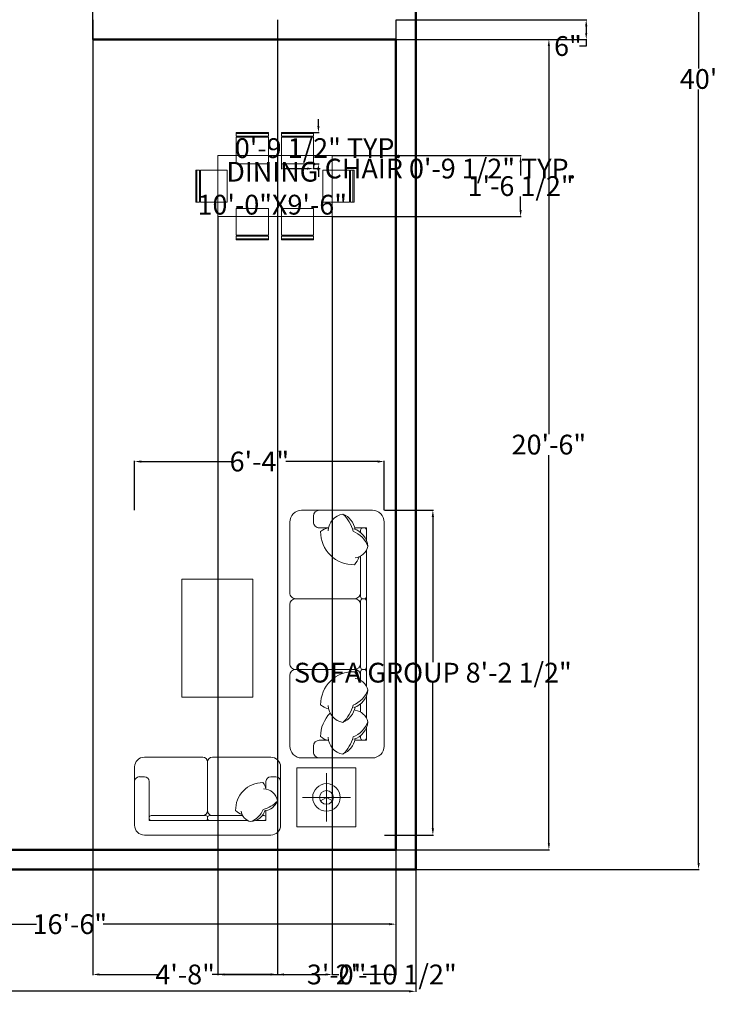
# Model space of a CAD drawing. Units: inches. Extents: x 20 to 32681, y 45 to 3082.
# Tile 2 of 5: x 301 to 512, y 45 to 344. Entities that reach past the tile are written whole.
import ezdxf

# ---------------------------------------------------------------- set-up
doc = ezdxf.new("R2010")
doc.units = ezdxf.units.IN
doc.header["$MEASUREMENT"] = 0
for name, color, linetype, lineweight in [('A-ANNO-DIMS', 2, 'Continuous', 18), ('A-AREA-IDEN', 7, 'Continuous', 25), ('A-FLOR-STRS', 3, 'Continuous', 25), ('A-FURN', 8, 'Continuous', 18), ('A-WALL', 7, 'Continuous', 50)]:
    doc.layers.add(name, color=color, linetype=linetype, lineweight=lineweight)
doc.styles.get("Standard").update_dxf_attribs({"font": 'arial.ttf'})
doc.dimstyles.get("Standard").update_dxf_attribs({"dimtxt": 6, "dimasz": 2, "dimexe": 0.18, "dimexo": 0.0625, "dimgap": 0.09, "dimtad": 0, "dimtih": 1, "dimtoh": 1, "dimdec": 0, "dimzin": 0, "dimdsep": 46, "dimlunit": 4, "dimtxsty": 'Standard', "dimcen": 0.09, "dimadec": 0, "dimazin": 0, "dimtfac": 1, "dimtdec": 0, "dimtofl": 0, "dimtmove": 0, "dimatfit": 3, "dimfxl": 1, "dimtolj": 1, "dimtzin": 0, "dimarcsym": 0})

# ---------------------------------------------------------------- blocks, each defined once
blk = doc.blocks.new('A$C17D461A9')
for p, q in [((2000, 3023.5), (100, 3023.5)), ((0, 2923.5), (0, 2323.5)), ((2100, 2323.5), (2100, 2923.5)), ((150, 2775.3), (150, 2873.5)), ((150, 2873.5), (255.2, 2873.5)), ((150, 2843.5), (150, 2853.5)), ((170, 2873.5), (255.2, 2873.5)), ((338.4, 2873.5), (1492.3, 2873.5)), ((338.4, 2873.5), (730, 2873.5)), ((750, 2853.5), (750, 2843.5)), ((750, 2853.5), (750, 2843.5)), ((1330, 2873.5), (770, 2873.5)), ((1350, 2843.5), (1350, 2853.5)), ((1350, 2853.5), (1350, 2843.5)), ((1492.3, 2873.5), (1370, 2873.5)), ((1575.5, 2873.5), (1761.6, 2873.5)), ((1761.6, 2873.5), (1575.5, 2873.5)), ((1930, 2873.5), (1844.8, 2873.5)), ((1844.8, 2873.5), (1950, 2873.5)), ((1950, 2873.5), (1950, 2775.3)), ((1950, 2843.5), (1950, 2853.5)), ((188.2, 2823.5), (170, 2823.5)), ((730, 2823.5), (388.7, 2823.5)), ((750, 2773.5), (750, 2273.5)), ((770, 2823.5), (1330, 2823.5)), ((1350, 2773.5), (1350, 2273.5)), ((1370, 2823.5), (1441.9, 2823.5)), ((1642.5, 2823.5), (1711.3, 2823.5)), ((1911.8, 2823.5), (1930, 2823.5)), ((2185, 2284.3), (2185, 2784.3)), ((2185, 2784.3), (2685, 2784.3)), ((2685, 2784.3), (2685, 2284.3)), ((2435, 2330.1), (2435, 2738.5)), ((150, 2473.5), (150, 2551)), ((1950, 2551), (1950, 2473.5)), ((2639.2, 2534.3), (2230.8, 2534.3)), ((2435, 2534.3), (2464.2, 2584.8)), ((2435, 2534.3), (2464.2, 2483.8)), ((50, 2423.5), (100, 2423.5)), ((2000, 2423.5), (2050, 2423.5)), ((2685, 2284.3), (2185, 2284.3)), ((100, 2223.5), (700, 2223.5)), ((800, 2223.5), (1300, 2223.5)), ((1400, 2223.5), (2000, 2223.5)), ((2671.6, 2144.9), (2176.6, 2144.9)), ((2259.1, 2062.4), (2259.1, 2103.6)), ((2094.1, 2062.4), (2094.1, 1567.4)), ((2364.3, 2021.1), (2300.3, 2021.1)), ((2549.3, 2021.1), (2630.3, 2021.1)), ((2589.1, 1989.6), (2589.1, 2004.6)), ((2605.6, 2021.1), (2613.8, 2021.1)), ((2630.3, 2021.1), (2630.3, 1934.3)), ((2630.3, 2004.6), (2630.3, 1934.3)), ((2754.1, 989.9), (2754.1, 2062.4)), ((2630.3, 1865.7), (2630.3, 1031.1)), ((2630.3, 1865.7), (2630.3, 1031.1)), ((2630.3, 1865.7), (2630.3, 1542.6)), ((2589.1, 1542.6), (2589.1, 1824.2)), ((2135.3, 1526.1), (2547.8, 1526.1)), ((2589.1, 1509.6), (2589.1, 1047.6)), ((2613.8, 1526.1), (2605.6, 1526.1)), ((2613.8, 1526.1), (2605.6, 1526.1)), ((2630.3, 1047.6), (2630.3, 1509.6)), ((2094.1, 1484.9), (2094.1, 989.9)), ((2630.3, 1031.1), (2300.3, 1031.1)), ((2630.3, 1031.1), (2300.3, 1031.1)), ((2605.6, 1031.1), (2613.8, 1031.1)), ((2259.1, 989.9), (2259.1, 948.6)), ((2259.1, 989.9), (2259.1, 948.6)), ((2176.6, 907.4), (2671.6, 907.4))]:
    blk.add_line(p, q)
blk.add_lwpolyline([(1585, 1308.5), (585, 1308.5), (585, 1908.5), (1585, 1908.5)], close=True)
for radius in [116.7, 58.3]:
    blk.add_circle((2435, 2534.3), radius)
for centre, radius, start, end in [((100, 2923.5), 100, 90, 180), ((2000, 2923.5), 100, 0, 90), ((170, 2853.5), 20, 90, 180), ((170, 2843.5), 20, 180, 270), ((320.4, 2716.2), 170.3, 94.53318, 162.72864), ((383.4, 2678.7), 220.9, 110.25938, 158.43175), ((275.1, 2759.5), 130.4, 7.76802, 75.89361), ((730, 2853.5), 20, 0, 90), ((730, 2843.5), 20, 270, 0), ((770, 2853.5), 20, 90, 180), ((770, 2843.5), 20, 180, 270), ((1330, 2853.5), 20, 0, 90), ((1330, 2843.5), 20, 270, 0), ((1370, 2853.5), 20, 90, 180), ((1370, 2843.5), 20, 180, 270), ((1555.5, 2759.5), 130.4, 104.10639, 172.23198), ((1447.3, 2678.7), 220.9, 21.56825, 69.74062), ((1510.3, 2716.2), 170.3, 17.27136, 85.46682), ((1824.9, 2759.5), 130.4, 104.10639, 172.23198), ((1716.6, 2678.7), 220.9, 21.56825, 69.74062), ((1779.6, 2716.2), 170.3, 17.27136, 85.46682), ((1930, 2853.5), 20, 0, 90), ((1930, 2843.5), 20, 270, 0), ((194.3, 2604), 176.9, 100.63867, 156.68485), ((247.1, 2475.1), 293.1, 103.64916, 137.26323), ((183.6, 2763.1), 278.1, 269.42107, 1.71498), ((348.3, 2656), 161.7, 45.50553, 73.22072), ((700, 2773.5), 50, 0, 90), ((800, 2773.5), 50, 90, 180), ((1300, 2773.5), 50, 0, 90), ((1400, 2773.5), 50, 90, 180), ((1647, 2763.1), 278.1, 178.28502, 270.57893), ((1482.4, 2656), 161.7, 106.77928, 134.49447), ((1583.5, 2475.1), 293.1, 42.73677, 76.35084), ((1636.4, 2604), 176.9, 23.31515, 79.36133), ((1852.9, 2475.1), 293.1, 42.73677, 76.35084), ((1905.7, 2604), 176.9, 23.31515, 79.36133), ((180.5, 2698.6), 150.7, 189.39285, 267.93283), ((1650.1, 2698.6), 150.7, 272.06717, 350.60715), ((1919.5, 2698.6), 150.7, 272.06717, 350.60715), ((262.4, 2563.4), 113.2, 186.29025, 223.8884), ((1568.3, 2563.4), 113.2, 316.1116, 353.70975), ((1916.4, 2763.1), 278.1, 225.28827, 270.57893), ((1837.6, 2563.4), 113.2, 316.1116, 353.70975), ((50, 2473.5), 50, 180, 270), ((100, 2473.5), 50, 270, 0), ((2000, 2473.5), 50, 180, 270), ((2050, 2473.5), 50, 270, 0), ((100, 2323.5), 100, 180, 270), ((700, 2273.5), 50, 270, 0), ((800, 2273.5), 50, 180, 270), ((1300, 2273.5), 50, 270, 0), ((1400, 2273.5), 50, 180, 270), ((2000, 2323.5), 100, 270, 0), ((2176.6, 2062.4), 82.5, 90, 180), ((2300.3, 2103.6), 41.2, 90, 180), ((2486, 1995.9), 124.4, 99.39285, 177.93283), ((2408, 1984.6), 146, 10.63867, 66.68485), ((2301.6, 1941), 241.8, 13.64916, 47.26323), ((2671.6, 2062.4), 82.5, 0, 90), ((2300.3, 2062.4), 41.2, 180, 270), ((2374.5, 1928.4), 93.4, 96.29025, 133.8884), ((2500.6, 1880.6), 140.5, 4.53318, 72.72864), ((2605.6, 2004.6), 16.5, 90, 180), ((2613.8, 2004.6), 16.5, 0, 90), ((2539.2, 1993.4), 229.5, 179.42107, 271.71498), ((2469.6, 1828.6), 182.2, 20.25938, 68.43175), ((2536.3, 1917.9), 107.6, 277.76802, 345.89361), ((2450.9, 1857.5), 133.4, 315.50553, 343.22072), ((2135.3, 1567.4), 41.2, 180, 270), ((2136, 1484.2), 41.9, 90.92597, 179.07403), ((2547.8, 1567.4), 41.2, 270, 0), ((2547.8, 1484.9), 41.2, 0, 90), ((2605.6, 1542.6), 16.5, 180, 270), ((2605.6, 1509.6), 16.5, 90, 180), ((2613.8, 1542.6), 16.5, 270, 0), ((2613.8, 1509.6), 16.5, 0, 90), ((2300.3, 989.9), 41.2, 90, 180), ((2300.3, 989.9), 41.2, 90, 180), ((2605.6, 1047.6), 16.5, 180, 270), ((2613.8, 1047.6), 16.5, 270, 0), ((2176.6, 989.9), 82.5, 180, 270), ((2300.3, 948.6), 41.3, 180, 270), ((2300.3, 948.6), 41.3, 180, 270), ((2671.6, 989.9), 82.5, 270, 0)]:
    blk.add_arc(centre, radius, start, end)
blk = doc.blocks.new('*D20')
at = {"layer": 'A-ANNO-DIMS', "color": 0, "lineweight": -2, "transparency": 16777216}
for p, q in [((216.79, 91.51), (216.79, 68.82)), ((414.79, 91.51), (414.79, 68.82)), ((218.79, 69), (305.68, 69)), ((412.79, 69), (325.9, 69))]:
    blk.add_line(p, q, dxfattribs=at)
at = {"layer": 'A-ANNO-DIMS', "color": 0, "transparency": 16777216}
for points in [[(218.79, 69.34), (218.79, 68.67), (216.79, 69)], [(412.79, 69.34), (412.79, 68.67), (414.79, 69)]]:
    blk.add_solid(points, dxfattribs=at)
at = {"layer": 'Defpoints', "color": 0, "transparency": 16777216}
for p in [(216.79, 91.58), (414.79, 91.58), (414.79, 69)]:
    blk.add_point(p, dxfattribs=at)
at = {"layer": 'A-ANNO-DIMS', "color": 0, "transparency": 16777216, "insert": (315.79, 69), "char_height": 6, "attachment_point": 5}
blk.add_mtext('\\A1;16\'-6"', dxfattribs=at)
blk = doc.blocks.new('*D21')
at = {"layer": 'A-ANNO-DIMS', "color": 0, "lineweight": -2, "transparency": 16777216}
for p, q in [((414.85, 337.58), (461.4, 337.58)), ((461.22, 335.58), (461.22, 217.73)), ((461.22, 93.58), (461.22, 211.42)), ((414.85, 91.58), (461.4, 91.58))]:
    blk.add_line(p, q, dxfattribs=at)
at = {"layer": 'A-ANNO-DIMS', "color": 0, "transparency": 16777216}
for points in [[(460.88, 335.58), (461.55, 335.58), (461.22, 337.58)], [(460.88, 93.58), (461.55, 93.58), (461.22, 91.58)]]:
    blk.add_solid(points, dxfattribs=at)
at = {"layer": 'Defpoints', "color": 0, "transparency": 16777216}
for p in [(414.79, 337.58), (461.22, 337.58), (414.79, 91.58)]:
    blk.add_point(p, dxfattribs=at)
at = {"layer": 'A-ANNO-DIMS', "color": 0, "transparency": 16777216, "insert": (461.22, 214.58), "char_height": 6, "attachment_point": 5}
blk.add_mtext('\\A1;20\'-6"', dxfattribs=at)
blk = doc.blocks.new('*D22')
at = {"layer": 'A-ANNO-DIMS', "color": 0, "lineweight": -2, "transparency": 16777216}
for p, q in [((414.85, 343.58), (472.74, 343.58)), ((472.56, 341.58), (472.56, 339.58)), ((414.85, 337.58), (472.74, 337.58)), ((472.56, 335.58), (470.56, 335.58)), ((472.56, 337.58), (472.56, 335.58))]:
    blk.add_line(p, q, dxfattribs=at)
at = {"layer": 'A-ANNO-DIMS', "color": 0, "transparency": 16777216}
for points in [[(472.23, 341.58), (472.89, 341.58), (472.56, 343.58)], [(472.23, 339.58), (472.89, 339.58), (472.56, 337.58)]]:
    blk.add_solid(points, dxfattribs=at)
at = {"layer": 'Defpoints', "color": 0, "transparency": 16777216}
for p in [(414.79, 343.58), (414.79, 337.58), (472.56, 337.58)]:
    blk.add_point(p, dxfattribs=at)
at = {"layer": 'A-ANNO-DIMS', "color": 0, "transparency": 16777216, "insert": (467, 335.58), "char_height": 6, "attachment_point": 5}
blk.add_mtext('\\A1;6"', dxfattribs=at)
blk = doc.blocks.new('*D27')
at = {"layer": 'A-ANNO-DIMS', "color": 0, "lineweight": -2, "transparency": 16777216}
for p, q in [((60.79, 85.51), (60.79, 48.43)), ((420.79, 85.51), (420.79, 48.43)), ((62.79, 48.61), (235.61, 48.61)), ((418.79, 48.61), (245.97, 48.61))]:
    blk.add_line(p, q, dxfattribs=at)
at = {"layer": 'A-ANNO-DIMS', "color": 0, "transparency": 16777216}
for points in [[(62.79, 48.94), (62.79, 48.27), (60.79, 48.61)], [(418.79, 48.94), (418.79, 48.27), (420.79, 48.61)]]:
    blk.add_solid(points, dxfattribs=at)
at = {"layer": 'Defpoints', "color": 0, "transparency": 16777216}
for p in [(60.79, 85.58), (420.79, 85.58), (420.79, 48.61)]:
    blk.add_point(p, dxfattribs=at)
at = {"layer": 'A-ANNO-DIMS', "color": 0, "transparency": 16777216, "insert": (240.79, 48.61), "char_height": 6, "attachment_point": 5}
blk.add_mtext("\\A1;30'", dxfattribs=at)
blk = doc.blocks.new('*D28')
at = {"layer": 'A-ANNO-DIMS', "color": 0, "lineweight": -2, "transparency": 16777216}
for p, q in [((420.85, 565.58), (506.85, 565.58)), ((506.67, 563.58), (506.67, 328.73)), ((506.67, 87.58), (506.67, 322.42)), ((420.85, 85.58), (506.85, 85.58))]:
    blk.add_line(p, q, dxfattribs=at)
at = {"layer": 'A-ANNO-DIMS', "color": 0, "transparency": 16777216}
for points in [[(506.34, 563.58), (507.01, 563.58), (506.67, 565.58)], [(506.34, 87.58), (507.01, 87.58), (506.67, 85.58)]]:
    blk.add_solid(points, dxfattribs=at)
at = {"layer": 'Defpoints', "color": 0, "transparency": 16777216}
for p in [(420.79, 565.58), (506.67, 565.58), (420.79, 85.58)]:
    blk.add_point(p, dxfattribs=at)
at = {"layer": 'A-ANNO-DIMS', "color": 0, "transparency": 16777216, "insert": (506.67, 325.58), "char_height": 6, "attachment_point": 5}
blk.add_mtext("\\A1;40'", dxfattribs=at)
blk = doc.blocks.new('CHAIR-DINING')
for p, q in [((9.73, 0.33), (0, 0.33)), ((0, 0.33), (0, -0.75)), ((0, 0), (9.73, 0)), ((9.73, -0.75), (9.73, 0.33)), ((0, -0.75), (9.73, -0.75)), ((0, -9.17), (0, -1.07)), ((0, -1.07), (9.73, -1.07)), ((9.73, -1.07), (9.73, -9.17)), ((9.73, -9.17), (0, -9.17))]:
    blk.add_line(p, q)
blk = doc.blocks.new('*D36')
at = {"layer": 'A-ANNO-DIMS', "color": 0, "lineweight": -2, "transparency": 16777216}
for p, q in [((411.27, 194.65), (426.18, 194.65)), ((426, 192.65), (426, 148.54)), ((426, 98.05), (426, 142.16)), ((411.27, 96.05), (426.18, 96.05))]:
    blk.add_line(p, q, dxfattribs=at)
at = {"layer": 'A-ANNO-DIMS', "color": 0, "transparency": 16777216}
for points in [[(425.66, 192.65), (426.33, 192.65), (426, 194.65)], [(425.66, 98.05), (426.33, 98.05), (426, 96.05)]]:
    blk.add_solid(points, dxfattribs=at)
at = {"layer": 'Defpoints', "color": 0, "transparency": 16777216}
for p in [(411.21, 194.65), (411.21, 96.05), (426, 96.05)]:
    blk.add_point(p, dxfattribs=at)
at = {"layer": 'A-ANNO-DIMS', "color": 0, "transparency": 16777216, "insert": (426, 145.35), "char_height": 6, "attachment_point": 5}
blk.add_mtext('\\A1;SOFA GROUP 8\'-2 1/2"', dxfattribs=at)
blk = doc.blocks.new('*D37')
at = {"layer": 'A-ANNO-DIMS', "color": 0, "lineweight": -2, "transparency": 16777216}
for p, q in [((335.45, 194.71), (335.45, 209.62)), ((337.45, 209.44), (365.25, 209.44)), ((409.21, 209.44), (381.41, 209.44)), ((411.21, 194.71), (411.21, 209.62))]:
    blk.add_line(p, q, dxfattribs=at)
at = {"layer": 'A-ANNO-DIMS', "color": 0, "transparency": 16777216}
for points in [[(337.45, 209.77), (337.45, 209.1), (335.45, 209.44)], [(409.21, 209.77), (409.21, 209.1), (411.21, 209.44)]]:
    blk.add_solid(points, dxfattribs=at)
at = {"layer": 'Defpoints', "color": 0, "transparency": 16777216}
for p in [(411.21, 209.44), (335.45, 194.65), (411.21, 194.65)]:
    blk.add_point(p, dxfattribs=at)
at = {"layer": 'A-ANNO-DIMS', "color": 0, "transparency": 16777216, "insert": (373.33, 209.44), "char_height": 6, "attachment_point": 5}
blk.add_mtext('\\A1;6\'-4"', dxfattribs=at)
blk = doc.blocks.new('*D38')
at = {"layer": 'A-ANNO-DIMS', "color": 0, "lineweight": -2, "transparency": 16777216}
for p, q in [((380.06, 299.77), (380.06, 298.2)), ((389.79, 299.77), (389.79, 298.2)), ((382.06, 298.38), (387.79, 298.38)), ((389.79, 298.38), (391.79, 298.38))]:
    blk.add_line(p, q, dxfattribs=at)
at = {"layer": 'A-ANNO-DIMS', "color": 0, "transparency": 16777216}
for points in [[(382.06, 298.71), (382.06, 298.04), (380.06, 298.38)], [(387.79, 298.71), (387.79, 298.04), (389.79, 298.38)]]:
    blk.add_solid(points, dxfattribs=at)
at = {"layer": 'Defpoints', "color": 0, "transparency": 16777216}
for p in [(380.06, 299.84), (389.79, 299.84), (389.79, 298.38)]:
    blk.add_point(p, dxfattribs=at)
at = {"layer": 'A-ANNO-DIMS', "color": 0, "transparency": 16777216, "insert": (431.32, 298.38), "char_height": 6, "attachment_point": 5}
blk.add_mtext('\\A1;CHAIR 0\'-9 1/2" TYP.', dxfattribs=at)
blk = doc.blocks.new('*D39')
at = {"layer": 'A-ANNO-DIMS', "color": 0, "lineweight": -2, "transparency": 16777216}
for p, q in [((391.25, 311.34), (391.25, 313.34)), ((389.85, 309.34), (391.43, 309.34)), ((389.85, 299.84), (391.43, 299.84)), ((391.25, 297.84), (391.25, 295.84))]:
    blk.add_line(p, q, dxfattribs=at)
at = {"layer": 'A-ANNO-DIMS', "color": 0, "transparency": 16777216}
for points in [[(390.91, 311.34), (391.58, 311.34), (391.25, 309.34)], [(390.91, 297.84), (391.58, 297.84), (391.25, 299.84)]]:
    blk.add_solid(points, dxfattribs=at)
at = {"layer": 'Defpoints', "color": 0, "transparency": 16777216}
for p in [(389.79, 309.34), (391.25, 309.34), (389.79, 299.84)]:
    blk.add_point(p, dxfattribs=at)
at = {"layer": 'A-ANNO-DIMS', "color": 0, "transparency": 16777216, "insert": (391.25, 304.59), "char_height": 6, "attachment_point": 5}
blk.add_mtext('\\A1;0\'-9 1/2" TYP.', dxfattribs=at)
blk = doc.blocks.new('*D44')
at = {"layer": 'A-ANNO-DIMS', "color": 0, "lineweight": -2, "transparency": 16777216}
for p, q in [((322.79, 343.51), (322.79, 53.55)), ((378.79, 343.51), (378.79, 53.55)), ((324.79, 53.73), (342.61, 53.73)), ((376.79, 53.73), (358.98, 53.73))]:
    blk.add_line(p, q, dxfattribs=at)
at = {"layer": 'A-ANNO-DIMS', "color": 0, "transparency": 16777216}
for points in [[(324.79, 54.06), (324.79, 53.39), (322.79, 53.73)], [(376.79, 54.06), (376.79, 53.39), (378.79, 53.73)]]:
    blk.add_solid(points, dxfattribs=at)
at = {"layer": 'Defpoints', "color": 0, "transparency": 16777216}
for p in [(322.79, 343.58), (378.79, 343.58), (378.79, 53.73)]:
    blk.add_point(p, dxfattribs=at)
at = {"layer": 'A-ANNO-DIMS', "color": 0, "transparency": 16777216, "insert": (350.79, 53.73), "char_height": 6, "attachment_point": 5}
blk.add_mtext('\\A1;4\'-8"', dxfattribs=at)
blk = doc.blocks.new('*D45')
at = {"layer": 'A-ANNO-DIMS', "color": 0, "lineweight": -2, "transparency": 16777216}
for p, q in [((378.79, 343.51), (378.79, 53.55)), ((414.79, 343.51), (414.79, 53.55)), ((380.79, 53.73), (388.73, 53.73)), ((412.79, 53.73), (404.85, 53.73))]:
    blk.add_line(p, q, dxfattribs=at)
at = {"layer": 'A-ANNO-DIMS', "color": 0, "transparency": 16777216}
for points in [[(380.79, 54.06), (380.79, 53.39), (378.79, 53.73)], [(412.79, 54.06), (412.79, 53.39), (414.79, 53.73)]]:
    blk.add_solid(points, dxfattribs=at)
at = {"layer": 'Defpoints', "color": 0, "transparency": 16777216}
for p in [(378.79, 343.58), (414.79, 343.58), (414.79, 53.73)]:
    blk.add_point(p, dxfattribs=at)
at = {"layer": 'A-ANNO-DIMS', "color": 0, "transparency": 16777216, "insert": (396.79, 53.73), "char_height": 6, "attachment_point": 5}
blk.add_mtext('\\A1;3\'-0"', dxfattribs=at)
blk = doc.blocks.new('*D48')
at = {"layer": 'A-ANNO-DIMS', "color": 0, "lineweight": -2, "transparency": 16777216}
for p, q in [((360.69, 283.73), (360.69, 53.55)), ((395.43, 283.73), (395.43, 53.55)), ((362.69, 53.73), (393.43, 53.73)), ((395.43, 53.73), (397.43, 53.73))]:
    blk.add_line(p, q, dxfattribs=at)
at = {"layer": 'A-ANNO-DIMS', "color": 0, "transparency": 16777216}
for points in [[(362.69, 54.06), (362.69, 53.39), (360.69, 53.73)], [(393.43, 54.06), (393.43, 53.39), (395.43, 53.73)]]:
    blk.add_solid(points, dxfattribs=at)
at = {"layer": 'Defpoints', "color": 0, "transparency": 16777216}
for p in [(360.69, 283.79), (395.43, 283.79), (395.43, 53.73)]:
    blk.add_point(p, dxfattribs=at)
at = {"layer": 'A-ANNO-DIMS', "color": 0, "transparency": 16777216, "insert": (414.86, 53.73), "char_height": 6, "attachment_point": 5}
blk.add_mtext('\\A1;2\'-10 1/2"', dxfattribs=at)
blk = doc.blocks.new('*D49')
at = {"layer": 'A-ANNO-DIMS', "color": 0, "lineweight": -2, "transparency": 16777216}
for p, q in [((395.49, 302.32), (452.82, 302.32)), ((452.64, 300.32), (452.64, 296.25)), ((452.64, 285.79), (452.64, 289.86)), ((395.49, 283.79), (452.82, 283.79))]:
    blk.add_line(p, q, dxfattribs=at)
at = {"layer": 'A-ANNO-DIMS', "color": 0, "transparency": 16777216}
for points in [[(452.31, 300.32), (452.97, 300.32), (452.64, 302.32)], [(452.31, 285.79), (452.97, 285.79), (452.64, 283.79)]]:
    blk.add_solid(points, dxfattribs=at)
at = {"layer": 'Defpoints', "color": 0, "transparency": 16777216}
for p in [(395.43, 302.32), (395.43, 283.79), (452.64, 283.79)]:
    blk.add_point(p, dxfattribs=at)
at = {"layer": 'A-ANNO-DIMS', "color": 0, "transparency": 16777216, "insert": (452.64, 293.06), "char_height": 6, "attachment_point": 5}
blk.add_mtext('\\A1;1\'-6 1/2"', dxfattribs=at)

msp = doc.modelspace()

# ---------------------------------------------------------------- linework, layer by layer
at = {"layer": 'A-FLOR-STRS'}
msp.add_line((322.79, 337.58), (322.79, 373.58), dxfattribs=at)
at = {"layer": 'A-FURN'}
for p, q in [((360.69, 283.79), (360.69, 302.32)), ((360.69, 302.32), (395.43, 302.32)), ((395.43, 302.32), (395.43, 283.79)), ((395.43, 283.79), (360.69, 283.79))]:
    msp.add_line(p, q, dxfattribs=at)
at = {"layer": 'A-WALL'}
for p, q in [((420.79, 85.58), (420.79, 565.58)), ((322.79, 337.58), (414.79, 337.58)), ((414.79, 91.58), (414.79, 337.58)), ((252.79, 91.58), (414.79, 91.58)), ((252.79, 85.58), (420.79, 85.58))]:
    msp.add_line(p, q, dxfattribs=at)

# ---------------------------------------------------------------- block references
at = {"layer": 'A-FURN'}
for p in [(366.33, 309.01), (380.06, 309.01)]:
    msp.add_blockref('CHAIR-DINING', p, dxfattribs=at)
for p, rotation in [((354.37, 288.17), 90.00000000000662), ((401.75, 297.89), 270.0000000000051), ((376.06, 277.1), 180), ((389.79, 277.1), 180)]:
    msp.add_blockref('CHAIR-DINING', p, dxfattribs=dict(at, rotation=rotation))
at = {"layer": 'A-FURN', "xscale": 0.0357995907885528, "yscale": 0.0357995907885528, "zscale": 0.0357995907885528, "rotation": 270}
msp.add_blockref('A$C17D461A9', (302.97, 194.65), dxfattribs=at)

# ---------------------------------------------------------------- texts
at = {"layer": 'A-AREA-IDEN', "insert": (334.92, 300.42), "char_height": 6, "attachment_point": 1}
msp.add_mtext_dynamic_manual_height_columns('\\pxqc;DINING\\P10\'-0"X9\'-6"', width=84.6469, gutter_width=30, heights=[0], dxfattribs=at)

# ---------------------------------------------------------------- dimensions: what is measured, and where the dimension line sits
at = {"layer": 'A-ANNO-DIMS'}
for base, p1, p2, override, picture, middle in [((506.67, 565.58), (420.79, 85.58), (420.79, 565.58), {"dimclrd": 0, "dimclre": 0, "dimclrt": 0}, '*D28', (506.67, 325.58)), ((472.56, 337.58), (414.79, 343.58), (414.79, 337.58), {"dimclrd": 0, "dimclre": 0, "dimclrt": 0}, '*D22', (467, 335.58)), ((461.22, 337.58), (414.79, 91.58), (414.79, 337.58), {"dimclrd": 0, "dimclre": 0, "dimclrt": 0}, '*D21', (461.22, 214.58)), ((452.64, 283.79), (395.43, 302.32), (395.43, 283.79), {"dimdec": 1, "dimlfac": 1, "dimrnd": 0, "dimzin": 1, "dimdsep": 46, "dimlunit": 4, "dimfrac": 2}, '*D49', (452.64, 293.06))]:
    dim = msp.add_linear_dim(base=base, p1=p1, p2=p2, angle=90, dimstyle='Standard', override=override, dxfattribs=at)
    dim.commit()
    dim.dimension.update_dxf_attribs({"geometry": picture, "text_midpoint": middle})
for base, p1, p2, override, picture, middle in [((378.79, 53.73), (322.79, 343.58), (378.79, 343.58), {"dimdec": 1, "dimlfac": 1, "dimrnd": 0, "dimzin": 1, "dimdsep": 46, "dimlunit": 4, "dimfrac": 2}, '*D44', (350.79, 53.73)), ((414.79, 53.73), (378.79, 343.58), (414.79, 343.58), {"dimdec": 1, "dimlfac": 1, "dimrnd": 0, "dimzin": 1, "dimdsep": 46, "dimlunit": 4, "dimfrac": 2}, '*D45', (396.79, 53.73)), ((395.43, 53.73), (360.69, 283.79), (395.43, 283.79), {"dimdec": 1, "dimlfac": 1, "dimrnd": 0, "dimzin": 1, "dimdsep": 46, "dimlunit": 4, "dimfrac": 2}, '*D48', (414.86, 53.73)), ((411.21, 209.44), (335.45, 194.65), (411.21, 194.65), {"dimdec": 1, "dimlfac": 1, "dimrnd": 0, "dimzin": 1, "dimdsep": 46, "dimlunit": 4, "dimfrac": 2}, '*D37', (373.33, 209.44)), ((414.79, 69), (216.79, 91.58), (414.79, 91.58), {"dimclrd": 0, "dimclre": 0, "dimclrt": 0}, '*D20', (315.79, 69)), ((420.79, 48.61), (60.79, 85.58), (420.79, 85.58), {"dimclrd": 0, "dimclre": 0, "dimclrt": 0}, '*D27', (240.79, 48.61))]:
    dim = msp.add_linear_dim(base=base, p1=p1, p2=p2, dimstyle='Standard', override=override, dxfattribs=at)
    dim.commit()
    dim.dimension.update_dxf_attribs({"geometry": picture, "text_midpoint": middle})
for base, p1, p2, angle, text, picture, middle in [((391.25, 309.34), (389.79, 299.84), (389.79, 309.34), 90, '<> TYP.', '*D39', (391.25, 304.59)), ((426, 96.05), (411.21, 194.65), (411.21, 96.05), 270, 'SOFA GROUP <>', '*D36', (426, 145.35))]:
    dim = msp.add_linear_dim(base=base, p1=p1, p2=p2, angle=angle, text=text, dimstyle='Standard', override={"dimdec": 1, "dimlfac": 1, "dimrnd": 0, "dimzin": 1, "dimdsep": 46, "dimlunit": 4, "dimfrac": 2}, dxfattribs=at)
    dim.commit()
    dim.dimension.update_dxf_attribs({"geometry": picture, "text_midpoint": middle})
dim = msp.add_linear_dim(base=(389.79, 298.38), p1=(380.06, 299.84), p2=(389.79, 299.84), text='CHAIR <> TYP.', dimstyle='Standard', override={"dimdec": 1, "dimlfac": 1, "dimrnd": 0, "dimzin": 1, "dimdsep": 46, "dimlunit": 4, "dimfrac": 2}, dxfattribs=at)
dim.commit()
dim.dimension.update_dxf_attribs({"geometry": '*D38', "text_midpoint": (431.32, 298.38)})

doc.saveas('drawing.dxf')
